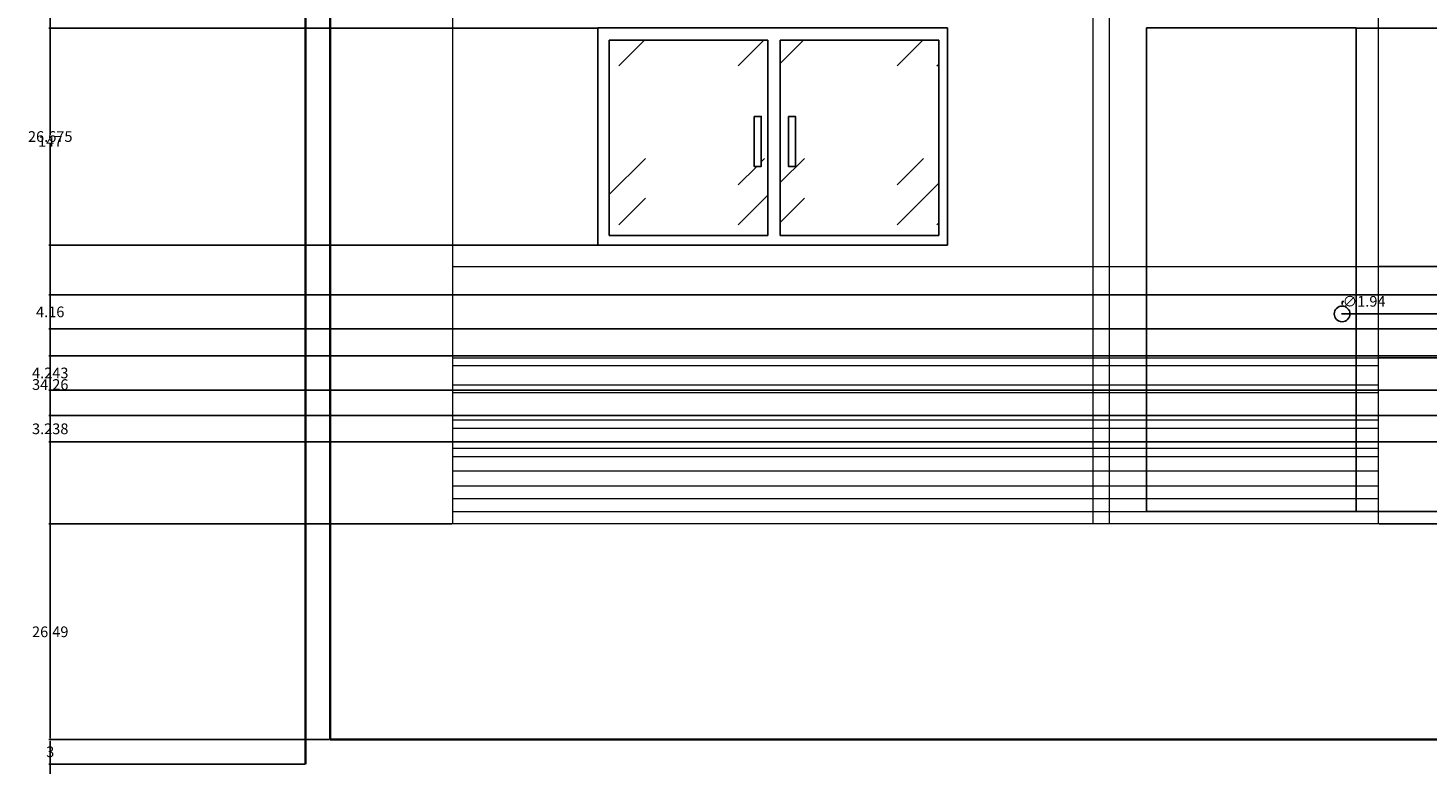
# Model space of a CAD drawing. Units: inches. Extents: x 30 to 515, y 94 to 489.
# Tile 2 of 7: x 30 to 202, y 266 to 356. Entities that reach past the tile are written whole.
import ezdxf

# ---------------------------------------------------------------- set-up
doc = ezdxf.new("R2010")
doc.units = ezdxf.units.IN
doc.header["$MEASUREMENT"] = 0
for name, color, linetype, lineweight in [('A-ANNO-DIMS', 2, 'Continuous', 18), ('A-DOOR', 4, 'Continuous', 25), ('A-FLOR-HRAL', 3, 'Continuous', 18), ('A-GLAZ', 4, 'Continuous', 25), ('A-GLAZ-PATT', 8, 'Continuous', 13), ('A-WALL', 7, 'Continuous', 35)]:
    doc.layers.add(name, color=color, linetype=linetype, lineweight=lineweight)
doc.styles.get("Standard").update_dxf_attribs({"font": 'arial.ttf'})
doc.dimstyles.get("Standard").update_dxf_attribs({"dimtxt": 1.3125, "dimasz": 0.18, "dimexe": 0.18, "dimexo": 0.0625, "dimgap": 0.09, "dimtad": 0, "dimtih": 1, "dimtoh": 1, "dimdec": 4, "dimzin": 0, "dimdsep": 46, "dimlunit": 4, "dimtxsty": 'Standard', "dimcen": 0.09, "dimadec": 0, "dimazin": 0, "dimtfac": 1, "dimtdec": 4, "dimtofl": 0, "dimtmove": 0, "dimatfit": 3, "dimfxl": 1, "dimtolj": 1, "dimtzin": 0, "dimarcsym": 0})

# ---------------------------------------------------------------- blocks, each defined once
blk = doc.blocks.new('*D24')
at = {"layer": 'A-ANNO-DIMS', "color": 0, "lineweight": -2, "transparency": 16777216}
for p, q in [((66.95, 268.53), (32.48, 268.53)), ((32.66, 268.35), (32.66, 237.07)), ((32.66, 204.27), (32.66, 235.55)), ((120.93, 204.09), (32.48, 204.09))]:
    blk.add_line(p, q, dxfattribs=at)
at = {"layer": 'A-ANNO-DIMS', "color": 0, "transparency": 16777216}
for points in [[(32.63, 268.35), (32.69, 268.35), (32.66, 268.53)], [(32.63, 204.27), (32.69, 204.27), (32.66, 204.09)]]:
    blk.add_solid(points, dxfattribs=at)
at = {"layer": 'Defpoints', "color": 0, "transparency": 16777216}
for p in [(32.66, 268.53), (67.02, 268.53), (120.99, 204.09)]:
    blk.add_point(p, dxfattribs=at)
at = {"layer": 'A-ANNO-DIMS', "color": 0, "transparency": 16777216, "insert": (32.66, 236.31), "char_height": 1.312, "attachment_point": 5}
blk.add_mtext('\\A1;64.43', dxfattribs=at)
blk = doc.blocks.new('*D25')
at = {"layer": 'A-ANNO-DIMS', "color": 0, "lineweight": -2, "transparency": 16777216}
for p, q in [((66.95, 415.53), (32.48, 415.53)), ((32.66, 415.35), (32.66, 342.78)), ((32.66, 268.71), (32.66, 341.28)), ((66.95, 268.53), (32.48, 268.53))]:
    blk.add_line(p, q, dxfattribs=at)
at = {"layer": 'A-ANNO-DIMS', "color": 0, "transparency": 16777216}
for points in [[(32.63, 415.35), (32.69, 415.35), (32.66, 415.53)], [(32.63, 268.71), (32.69, 268.71), (32.66, 268.53)]]:
    blk.add_solid(points, dxfattribs=at)
at = {"layer": 'Defpoints', "color": 0, "transparency": 16777216}
for p in [(32.66, 415.53), (67.02, 415.53), (67.02, 268.53)]:
    blk.add_point(p, dxfattribs=at)
at = {"layer": 'A-ANNO-DIMS', "color": 0, "transparency": 16777216, "insert": (32.66, 342.03), "char_height": 1.312, "attachment_point": 5}
blk.add_mtext('\\A1;147', dxfattribs=at)
blk = doc.blocks.new('*D49')
at = {"layer": 'A-ANNO-DIMS', "color": 0, "lineweight": -2, "transparency": 16777216}
for p, q in [((66.95, 268.53), (32.48, 268.53)), ((32.66, 268.35), (32.66, 267.79)), ((63.95, 265.53), (32.48, 265.53)), ((32.66, 265.71), (32.66, 266.27))]:
    blk.add_line(p, q, dxfattribs=at)
at = {"layer": 'A-ANNO-DIMS', "color": 0, "transparency": 16777216}
for points in [[(32.63, 268.35), (32.69, 268.35), (32.66, 268.53)], [(32.63, 265.71), (32.69, 265.71), (32.66, 265.53)]]:
    blk.add_solid(points, dxfattribs=at)
at = {"layer": 'Defpoints', "color": 0, "transparency": 16777216}
for p in [(32.66, 268.53), (67.02, 268.53), (64.02, 265.53)]:
    blk.add_point(p, dxfattribs=at)
at = {"layer": 'A-ANNO-DIMS', "color": 0, "transparency": 16777216, "insert": (32.66, 267.03), "char_height": 1.312, "attachment_point": 5}
blk.add_mtext('\\A1;3', dxfattribs=at)
blk = doc.blocks.new('*D50')
at = {"layer": 'A-ANNO-DIMS', "color": 0, "lineweight": -2, "transparency": 16777216}
for p, q in [((82.01, 295.02), (32.48, 295.02)), ((32.66, 294.84), (32.66, 282.53)), ((32.66, 268.71), (32.66, 281.01)), ((66.95, 268.53), (32.48, 268.53))]:
    blk.add_line(p, q, dxfattribs=at)
at = {"layer": 'A-ANNO-DIMS', "color": 0, "transparency": 16777216}
for points in [[(32.63, 294.84), (32.69, 294.84), (32.66, 295.02)], [(32.63, 268.71), (32.69, 268.71), (32.66, 268.53)]]:
    blk.add_solid(points, dxfattribs=at)
at = {"layer": 'Defpoints', "color": 0, "transparency": 16777216}
for p in [(32.66, 295.02), (82.07, 295.02), (67.02, 268.53)]:
    blk.add_point(p, dxfattribs=at)
at = {"layer": 'A-ANNO-DIMS', "color": 0, "transparency": 16777216, "insert": (32.66, 281.77), "char_height": 1.312, "attachment_point": 5}
blk.add_mtext('\\A1;26.49', dxfattribs=at)
blk = doc.blocks.new('*D51')
at = {"layer": 'A-ANNO-DIMS', "color": 0, "lineweight": -2, "transparency": 16777216}
for p, q in [((99.83, 329.28), (32.48, 329.28)), ((32.66, 329.1), (32.66, 312.91)), ((32.66, 295.2), (32.66, 311.39)), ((82.01, 295.02), (32.48, 295.02))]:
    blk.add_line(p, q, dxfattribs=at)
at = {"layer": 'A-ANNO-DIMS', "color": 0, "transparency": 16777216}
for points in [[(32.63, 329.1), (32.69, 329.1), (32.66, 329.28)], [(32.63, 295.2), (32.69, 295.2), (32.66, 295.02)]]:
    blk.add_solid(points, dxfattribs=at)
at = {"layer": 'Defpoints', "color": 0, "transparency": 16777216}
for p in [(32.66, 329.28), (99.9, 329.28), (82.07, 295.02)]:
    blk.add_point(p, dxfattribs=at)
at = {"layer": 'A-ANNO-DIMS', "color": 0, "transparency": 16777216, "insert": (32.66, 312.15), "char_height": 1.312, "attachment_point": 5}
blk.add_mtext('\\A1;34.26', dxfattribs=at)
blk = doc.blocks.new('*D52')
at = {"layer": 'A-ANNO-DIMS', "color": 0, "lineweight": -2, "transparency": 16777216}
for p, q in [((99.83, 355.95), (32.48, 355.95)), ((32.66, 355.77), (32.66, 343.38)), ((32.66, 329.46), (32.66, 341.86)), ((99.83, 329.28), (32.48, 329.28))]:
    blk.add_line(p, q, dxfattribs=at)
at = {"layer": 'A-ANNO-DIMS', "color": 0, "transparency": 16777216}
for points in [[(32.63, 355.77), (32.69, 355.77), (32.66, 355.95)], [(32.63, 329.46), (32.69, 329.46), (32.66, 329.28)]]:
    blk.add_solid(points, dxfattribs=at)
at = {"layer": 'Defpoints', "color": 0, "transparency": 16777216}
for p in [(32.66, 355.95), (99.9, 355.95), (99.9, 329.28)]:
    blk.add_point(p, dxfattribs=at)
at = {"layer": 'A-ANNO-DIMS', "color": 0, "transparency": 16777216, "insert": (32.66, 342.62), "char_height": 1.312, "attachment_point": 5}
blk.add_mtext('\\A1;26.675', dxfattribs=at)
blk = doc.blocks.new('*D59')
at = {"layer": 'A-ANNO-DIMS', "color": 0, "lineweight": -2, "transparency": 16777216}
for p, q in [((193.04, 296.55), (512.17, 296.55)), ((511.99, 296.73), (511.99, 296.91)), ((195.76, 295.02), (512.17, 295.02)), ((511.99, 294.84), (511.99, 294.66))]:
    blk.add_line(p, q, dxfattribs=at)
at = {"layer": 'A-ANNO-DIMS', "color": 0, "transparency": 16777216}
for points in [[(511.96, 296.73), (512.02, 296.73), (511.99, 296.55)], [(511.96, 294.84), (512.02, 294.84), (511.99, 295.02)]]:
    blk.add_solid(points, dxfattribs=at)
at = {"layer": 'Defpoints', "color": 0, "transparency": 16777216}
for p in [(192.98, 296.55), (511.99, 296.55), (195.7, 295.02)]:
    blk.add_point(p, dxfattribs=at)
at = {"layer": 'A-ANNO-DIMS', "color": 0, "transparency": 16777216, "insert": (511.99, 295.78), "char_height": 1.312, "attachment_point": 5}
blk.add_mtext('\\A1;1.53', dxfattribs=at)
blk = doc.blocks.new('*D60')
at = {"layer": 'A-ANNO-DIMS', "color": 0, "lineweight": -2, "transparency": 16777216}
for p, q in [((191.31, 320.83), (512.17, 320.83)), ((511.99, 320.65), (511.99, 309.45)), ((511.99, 296.73), (511.99, 307.93)), ((193.04, 296.55), (512.17, 296.55))]:
    blk.add_line(p, q, dxfattribs=at)
at = {"layer": 'A-ANNO-DIMS', "color": 0, "transparency": 16777216}
for points in [[(511.96, 320.65), (512.02, 320.65), (511.99, 320.83)], [(511.96, 296.73), (512.02, 296.73), (511.99, 296.55)]]:
    blk.add_solid(points, dxfattribs=at)
at = {"layer": 'Defpoints', "color": 0, "transparency": 16777216}
for p in [(191.25, 320.83), (511.99, 320.83), (192.98, 296.55)]:
    blk.add_point(p, dxfattribs=at)
at = {"layer": 'A-ANNO-DIMS', "color": 0, "transparency": 16777216, "insert": (511.99, 308.69), "char_height": 1.312, "attachment_point": 5}
blk.add_mtext('\\A1;24.275', dxfattribs=at)
blk = doc.blocks.new('*D61')
at = {"layer": 'A-ANNO-DIMS', "color": 0, "lineweight": -2, "transparency": 16777216}
for p, q in [((193.04, 355.95), (512.17, 355.95)), ((511.99, 355.77), (511.99, 339.15)), ((511.99, 321.01), (511.99, 337.63)), ((191.31, 320.83), (512.17, 320.83))]:
    blk.add_line(p, q, dxfattribs=at)
at = {"layer": 'A-ANNO-DIMS', "color": 0, "transparency": 16777216}
for points in [[(511.96, 355.77), (512.02, 355.77), (511.99, 355.95)], [(511.96, 321.01), (512.02, 321.01), (511.99, 320.83)]]:
    blk.add_solid(points, dxfattribs=at)
at = {"layer": 'Defpoints', "color": 0, "transparency": 16777216}
for p in [(192.98, 355.95), (511.99, 355.95), (191.25, 320.83)]:
    blk.add_point(p, dxfattribs=at)
at = {"layer": 'A-ANNO-DIMS', "color": 0, "transparency": 16777216, "insert": (511.99, 338.39), "char_height": 1.312, "attachment_point": 5}
blk.add_mtext('\\A1;35.13', dxfattribs=at)
blk = doc.blocks.new('*D62')
at = {"layer": 'A-ANNO-DIMS', "color": 0, "lineweight": -2, "transparency": 16777216}
for p, q in [((195.76, 315.42), (512.17, 315.42)), ((511.99, 315.24), (511.99, 305.98)), ((511.99, 295.2), (511.99, 304.46)), ((195.76, 295.02), (512.17, 295.02))]:
    blk.add_line(p, q, dxfattribs=at)
at = {"layer": 'A-ANNO-DIMS', "color": 0, "transparency": 16777216}
for points in [[(511.96, 315.24), (512.02, 315.24), (511.99, 315.42)], [(511.96, 295.2), (512.02, 295.2), (511.99, 295.02)]]:
    blk.add_solid(points, dxfattribs=at)
at = {"layer": 'Defpoints', "color": 0, "transparency": 16777216}
for p in [(195.7, 315.42), (511.99, 315.42), (195.7, 295.02)]:
    blk.add_point(p, dxfattribs=at)
at = {"layer": 'A-ANNO-DIMS', "color": 0, "transparency": 16777216, "insert": (511.99, 305.22), "char_height": 1.312, "attachment_point": 5}
blk.add_mtext('\\A1;20.4', dxfattribs=at)
blk = doc.blocks.new('*D63')
at = {"layer": 'A-ANNO-DIMS', "color": 0, "lineweight": -2, "transparency": 16777216}
for p, q in [((195.76, 323.16), (512.17, 323.16)), ((511.99, 322.98), (511.99, 320.04)), ((511.99, 315.6), (511.99, 318.54)), ((195.76, 315.42), (512.17, 315.42))]:
    blk.add_line(p, q, dxfattribs=at)
at = {"layer": 'A-ANNO-DIMS', "color": 0, "transparency": 16777216}
for points in [[(511.96, 322.98), (512.02, 322.98), (511.99, 323.16)], [(511.96, 315.6), (512.02, 315.6), (511.99, 315.42)]]:
    blk.add_solid(points, dxfattribs=at)
at = {"layer": 'Defpoints', "color": 0, "transparency": 16777216}
for p in [(195.7, 323.16), (511.99, 323.16), (195.7, 315.42)]:
    blk.add_point(p, dxfattribs=at)
at = {"layer": 'A-ANNO-DIMS', "color": 0, "transparency": 16777216, "insert": (511.99, 319.29), "char_height": 1.312, "attachment_point": 5}
blk.add_mtext('\\A1;7.74', dxfattribs=at)
blk = doc.blocks.new('*D64')
at = {"layer": 'A-ANNO-DIMS', "color": 0, "lineweight": -2, "transparency": 16777216}
for p, q in [((195.76, 326.67), (512.17, 326.67)), ((511.99, 326.49), (511.99, 325.68)), ((195.76, 323.16), (512.17, 323.16)), ((511.99, 323.34), (511.99, 324.16))]:
    blk.add_line(p, q, dxfattribs=at)
at = {"layer": 'A-ANNO-DIMS', "color": 0, "transparency": 16777216}
for points in [[(511.96, 326.49), (512.02, 326.49), (511.99, 326.67)], [(511.96, 323.34), (512.02, 323.34), (511.99, 323.16)]]:
    blk.add_solid(points, dxfattribs=at)
at = {"layer": 'Defpoints', "color": 0, "transparency": 16777216}
for p in [(195.7, 326.67), (511.99, 326.67), (195.7, 323.16)]:
    blk.add_point(p, dxfattribs=at)
at = {"layer": 'A-ANNO-DIMS', "color": 0, "transparency": 16777216, "insert": (511.99, 324.92), "char_height": 1.312, "attachment_point": 5}
blk.add_mtext('\\A1;3.511', dxfattribs=at)
blk = doc.blocks.new('*D75')
at = {"layer": 'A-ANNO-DIMS', "color": 0, "lineweight": -2, "transparency": 16777216}
for p, q in [((380.57, 308.33), (32.48, 308.33)), ((32.66, 308.15), (32.66, 307.47)), ((32.66, 305.28), (32.66, 305.95)), ((380.57, 305.1), (32.48, 305.1))]:
    blk.add_line(p, q, dxfattribs=at)
at = {"layer": 'A-ANNO-DIMS', "color": 0, "transparency": 16777216}
for points in [[(32.63, 308.15), (32.69, 308.15), (32.66, 308.33)], [(32.63, 305.28), (32.69, 305.28), (32.66, 305.1)]]:
    blk.add_solid(points, dxfattribs=at)
at = {"layer": 'Defpoints', "color": 0, "transparency": 16777216}
for p in [(32.66, 308.33), (380.63, 308.33), (380.63, 305.1)]:
    blk.add_point(p, dxfattribs=at)
at = {"layer": 'A-ANNO-DIMS', "color": 0, "transparency": 16777216, "insert": (32.66, 306.71), "char_height": 1.312, "attachment_point": 5}
blk.add_mtext('\\A1;3.238', dxfattribs=at)
blk = doc.blocks.new('*D76')
at = {"layer": 'A-ANNO-DIMS', "color": 0, "lineweight": -2, "transparency": 16777216}
for p, q in [((380.57, 315.69), (32.48, 315.69)), ((32.66, 315.51), (32.66, 314.33)), ((32.66, 311.63), (32.66, 312.81)), ((380.57, 311.45), (32.48, 311.45))]:
    blk.add_line(p, q, dxfattribs=at)
at = {"layer": 'A-ANNO-DIMS', "color": 0, "transparency": 16777216}
for points in [[(32.63, 315.51), (32.69, 315.51), (32.66, 315.69)], [(32.63, 311.63), (32.69, 311.63), (32.66, 311.45)]]:
    blk.add_solid(points, dxfattribs=at)
at = {"layer": 'Defpoints', "color": 0, "transparency": 16777216}
for p in [(32.66, 315.69), (380.63, 315.69), (380.63, 311.45)]:
    blk.add_point(p, dxfattribs=at)
at = {"layer": 'A-ANNO-DIMS', "color": 0, "transparency": 16777216, "insert": (32.66, 313.57), "char_height": 1.312, "attachment_point": 5}
blk.add_mtext('\\A1;4.243', dxfattribs=at)
blk = doc.blocks.new('*D77')
at = {"layer": 'A-ANNO-DIMS', "color": 0, "lineweight": -2, "transparency": 16777216}
for p, q in [((380.57, 323.16), (32.48, 323.16)), ((32.66, 322.98), (32.66, 321.84)), ((32.66, 319.18), (32.66, 320.32)), ((380.57, 319), (32.48, 319))]:
    blk.add_line(p, q, dxfattribs=at)
at = {"layer": 'A-ANNO-DIMS', "color": 0, "transparency": 16777216}
for points in [[(32.63, 322.98), (32.69, 322.98), (32.66, 323.16)], [(32.63, 319.18), (32.69, 319.18), (32.66, 319)]]:
    blk.add_solid(points, dxfattribs=at)
at = {"layer": 'Defpoints', "color": 0, "transparency": 16777216}
for p in [(32.66, 323.16), (380.63, 323.16), (380.63, 319)]:
    blk.add_point(p, dxfattribs=at)
at = {"layer": 'A-ANNO-DIMS', "color": 0, "transparency": 16777216, "insert": (32.66, 321.08), "char_height": 1.312, "attachment_point": 5}
blk.add_mtext('\\A1;4.16', dxfattribs=at)
blk = doc.blocks.new('*D81')
at = {"layer": 'A-ANNO-DIMS', "color": 0, "lineweight": -2, "transparency": 16777216}
for p, q in [((191.27, 322.37), (191.26, 321.97)), ((191.45, 322.37), (191.27, 322.37)), ((191.16, 320.83), (191.34, 320.83)), ((191.25, 320.74), (191.25, 320.92))]:
    blk.add_line(p, q, dxfattribs=at)
at = {"layer": 'A-ANNO-DIMS', "color": 0, "transparency": 16777216}
blk.add_solid([(191.23, 321.97), (191.29, 321.97), (191.26, 321.79)], dxfattribs=at)
at = {"layer": 'Defpoints', "color": 0, "transparency": 16777216}
for p in [(191.26, 321.79), (191.24, 319.86)]:
    blk.add_point(p, dxfattribs=at)
at = {"layer": 'A-ANNO-DIMS', "color": 0, "transparency": 16777216, "insert": (193.95, 322.37), "char_height": 1.312, "attachment_point": 5}
blk.add_mtext('\\A1;∅1.94', dxfattribs=at)

msp = doc.modelspace()

# ---------------------------------------------------------------- hatches: boundary and pattern name
at = {"layer": 'A-GLAZ-PATT'}
h = msp.add_hatch(dxfattribs=at)
h.set_pattern_fill('GOST_GLASS', color=256, scale=2.3)
h.set_pattern_definition([(45, (0, 0), (19.51615, 0), [11.5, -16.1]), (45, (4.879, 0), (19.51615, 0), [4.6, -23]), (45, (0, 4.879), (19.51615, 0), [4.6, -23])])
h.paths.add_polyline_path([(141.7277, 354.4489), (122.2758, 354.4489), (122.2758, 330.4708), (141.7277, 330.4708)])
h.paths.add_polyline_path([(124.1475, 338.9533), (123.2785, 338.9533), (123.2785, 345.0981), (124.1475, 345.0981)], flags=16)
h.paths.add_polyline_path([(120.7384, 354.4489), (101.2865, 354.4489), (101.2865, 330.4708), (120.7384, 330.4708)])
h.paths.add_polyline_path([(119.0673, 338.9533), (119.0673, 345.0981), (119.9363, 345.0981), (119.9363, 338.9533)], flags=16)
h.paths.add_polyline_path([(159.5032, 242.6758), (123.7159, 242.6758), (123.7159, 205.8458), (159.5032, 205.8458)])
h.paths.add_polyline_path([(157.9822, 224.9831), (158.4447, 224.9831), (158.4447, 217.7871), (157.9822, 217.7871)], flags=16)
h.paths.add_polyline_path([(198.8424, 242.6758), (163.0551, 242.6758), (163.0551, 205.8458), (198.8424, 205.8458)])
h.paths.add_polyline_path([(164.8004, 224.9831), (164.8004, 217.7871), (164.3379, 217.7871), (164.3379, 224.9831)], flags=16)
h.paths.add_polyline_path([(389.467, 242.6758), (353.6798, 242.6758), (353.6798, 205.8458), (389.467, 205.8458)])
h.paths.add_polyline_path([(387.946, 224.9831), (388.4085, 224.9831), (388.4085, 217.7871), (387.946, 217.7871)], flags=16)
h.paths.add_polyline_path([(428.8062, 242.6758), (393.0189, 242.6758), (393.0189, 205.8458), (428.8062, 205.8458)])
h.paths.add_polyline_path([(394.7642, 224.9831), (394.7642, 217.7871), (394.3017, 217.7871), (394.3017, 224.9831)], flags=16)

# ---------------------------------------------------------------- linework, layer by layer
at = {"layer": 'A-DOOR'}
msp.add_lwpolyline([(167.2369, 355.9547), (192.9806, 355.9547), (192.9806, 296.551), (167.2369, 296.551)], close=True, dxfattribs=at)
msp.add_circle((191.2506, 320.8262), 0.9677, dxfattribs=at)
at = {"layer": 'A-FLOR-HRAL'}
for p, q in [((160.6442, 358.3247), (160.6442, 295.0176)), ((162.6442, 358.3247), (162.6442, 295.0176)), ((82.0736, 326.6711), (195.6952, 326.6711)), ((82.0736, 323.1601), (195.6952, 323.1601)), ((82.0736, 315.4195), (195.6952, 315.4195)), ((82.0736, 314.4748), (195.6952, 314.4748)), ((82.0736, 312.125), (195.6952, 312.125)), ((82.0736, 311.1803), (195.6952, 311.1803)), ((82.0736, 307.8112), (195.6952, 307.8112)), ((82.0736, 306.7888), (195.6952, 306.7888)), ((82.0736, 304.3296), (195.6952, 304.3296)), ((82.0736, 303.3072), (195.6952, 303.3072)), ((82.0736, 301.5437), (195.6952, 301.5437)), ((82.0736, 299.707), (195.6952, 299.707)), ((82.0736, 298.129), (195.6952, 298.129)), ((82.0736, 296.551), (195.6952, 296.551))]:
    msp.add_line(p, q, dxfattribs=at)
msp.add_lwpolyline([(82.0736, 358.3247), (195.6952, 358.3247), (195.6952, 295.0176), (82.0736, 295.0176)], close=True, dxfattribs=at)
at = {"layer": 'A-GLAZ'}
for points in [[(99.8974, 355.9547), (142.7973, 355.9547), (142.7973, 329.2795), (99.8974, 329.2795)], [(101.2865, 354.4489), (120.7384, 354.4489), (120.7384, 330.4708), (101.2865, 330.4708)], [(122.2758, 354.4489), (141.7277, 354.4489), (141.7277, 330.4708), (122.2758, 330.4708)], [(119.0673, 345.0981), (119.9363, 345.0981), (119.9363, 338.9533), (119.0673, 338.9533)], [(123.2785, 345.0981), (124.1475, 345.0981), (124.1475, 338.9533), (123.2785, 338.9533)]]:
    msp.add_lwpolyline(points, close=True, dxfattribs=at)
at = {"layer": 'A-WALL'}
for p, q in [((64.017, 268.5281), (64.017, 412.5281)), ((67.017, 268.5281), (67.017, 412.5281)), ((64.017, 268.5281), (64.017, 265.5281)), ((67.017, 268.5281), (448.0511, 268.5281))]:
    msp.add_line(p, q, dxfattribs=at)

# ---------------------------------------------------------------- dimensions: what is measured, and where the dimension line sits
at = {"layer": 'A-ANNO-DIMS'}
for base, p1, p2, override, picture, middle in [((32.6647, 415.5281), (67.017, 268.5281), (67.017, 415.5281), {"dimdec": 0, "dimlfac": 1, "dimrnd": 0, "dimzin": 0, "dimdsep": 46, "dimlunit": 2}, '*D25', (32.6647, 342.0281)), ((32.6647, 355.9547), (99.8974, 329.2795), (99.8974, 355.9547), {"dimdec": 3, "dimlfac": 1, "dimrnd": 0, "dimzin": 0, "dimdsep": 46, "dimlunit": 2}, '*D52', (32.6647, 342.6171)), ((511.9926, 355.9547), (191.2506, 320.8262), (192.9806, 355.9547), {"dimdec": 2, "dimlfac": 1, "dimrnd": 0, "dimzin": 0, "dimdsep": 46, "dimlunit": 2}, '*D61', (511.9926, 338.3905)), ((32.6647, 329.2795), (82.0736, 295.0176), (99.8974, 329.2795), {"dimdec": 2, "dimlfac": 1, "dimrnd": 0, "dimzin": 0, "dimdsep": 46, "dimlunit": 2}, '*D51', (32.6647, 312.1486)), ((511.9926, 326.6711), (195.6952, 323.1601), (195.6952, 326.6711), {"dimdec": 3, "dimlfac": 1, "dimrnd": 0, "dimzin": 0, "dimdsep": 46, "dimlunit": 2}, '*D64', (511.9926, 324.9156)), ((32.6647, 323.1601), (380.6303, 319.0036), (380.6303, 323.1601), {"dimdec": 2, "dimlfac": 1, "dimrnd": 0, "dimzin": 0, "dimdsep": 46, "dimlunit": 2}, '*D77', (32.6647, 321.0818)), ((511.9926, 323.1601), (195.6952, 315.4195), (195.6952, 323.1601), {"dimdec": 2, "dimlfac": 1, "dimrnd": 0, "dimzin": 0, "dimdsep": 46, "dimlunit": 2}, '*D63', (511.9926, 319.2898)), ((511.9926, 320.8262), (192.9806, 296.551), (191.2506, 320.8262), {"dimdec": 3, "dimlfac": 1, "dimrnd": 0, "dimzin": 0, "dimdsep": 46, "dimlunit": 2}, '*D60', (511.9926, 308.6886)), ((32.6647, 315.6935), (380.6303, 311.4502), (380.6303, 315.6935), {"dimdec": 3, "dimlfac": 1, "dimrnd": 0, "dimzin": 0, "dimdsep": 46, "dimlunit": 2}, '*D76', (32.6647, 313.5719)), ((511.9926, 315.4195), (195.6952, 295.0176), (195.6952, 315.4195), {"dimdec": 1, "dimlfac": 1, "dimrnd": 0, "dimzin": 0, "dimdsep": 46, "dimlunit": 2}, '*D62', (511.9926, 305.2186)), ((32.6647, 308.3335), (380.6303, 305.0952), (380.6303, 308.3335), {"dimdec": 3, "dimlfac": 1, "dimrnd": 0, "dimzin": 0, "dimdsep": 46, "dimlunit": 2}, '*D75', (32.6647, 306.7144)), ((511.9926, 296.551), (195.6952, 295.0176), (192.9806, 296.551), {"dimdec": 2, "dimlfac": 1, "dimrnd": 0, "dimzin": 0, "dimdsep": 46, "dimlunit": 2}, '*D59', (511.9926, 295.7843)), ((32.6647, 295.0176), (67.017, 268.5281), (82.0736, 295.0176), {"dimdec": 2, "dimlfac": 1, "dimrnd": 0, "dimzin": 0, "dimdsep": 46, "dimlunit": 2}, '*D50', (32.6647, 281.7728)), ((32.6647, 268.5281), (120.9898, 204.0939), (67.017, 268.5281), {"dimdec": 2, "dimlfac": 1, "dimrnd": 0, "dimzin": 0, "dimdsep": 46, "dimlunit": 2}, '*D24', (32.6647, 236.311)), ((32.6647, 268.5281), (64.017, 265.5281), (67.017, 268.5281), {"dimdec": 0, "dimlfac": 1, "dimrnd": 0, "dimzin": 0, "dimdsep": 46, "dimlunit": 2}, '*D49', (32.6647, 267.0281))]:
    dim = msp.add_linear_dim(base=base, p1=p1, p2=p2, angle=90, dimstyle='Standard', override=override, dxfattribs=at)
    dim.commit()
    dim.dimension.update_dxf_attribs({"geometry": picture, "text_midpoint": middle})
dim = msp.add_diameter_dim_2p(p1=(191.2408, 319.8586), p2=(191.2604, 321.7939), dimstyle='Standard', override={"dimdec": 2, "dimlfac": 1, "dimrnd": 0, "dimzin": 0, "dimdsep": 46, "dimlunit": 2}, dxfattribs=at)
dim.commit()
dim.dimension.update_dxf_attribs({"geometry": '*D81', "text_midpoint": (193.9523, 322.3745), "dimtype": 163})

doc.saveas('drawing.dxf')
